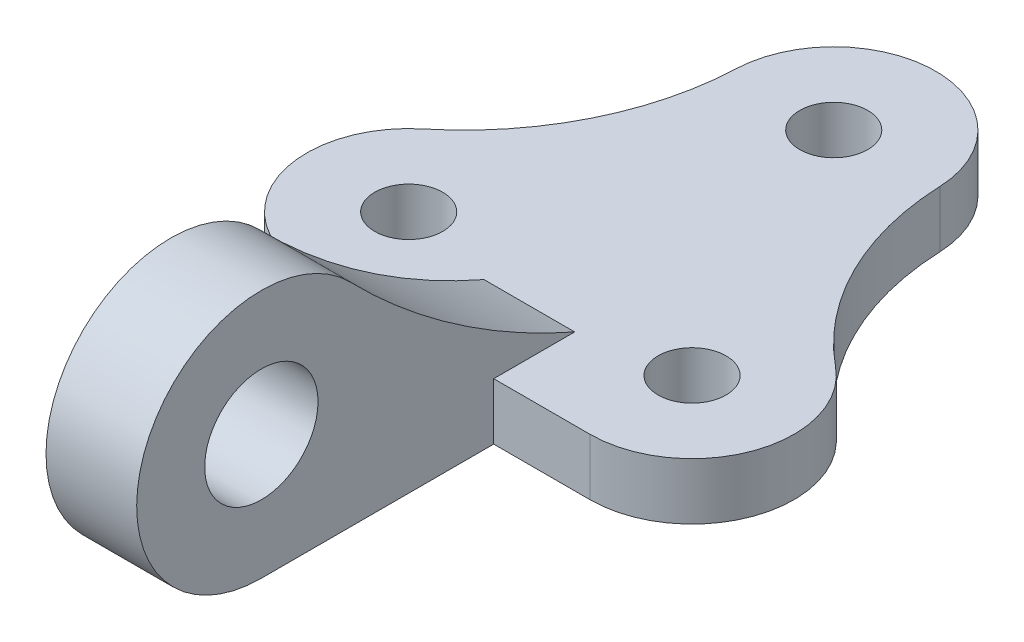
ISO-10303-21;
HEADER;
FILE_DESCRIPTION(('STEP AP214'),'2;1');
FILE_NAME('part.step','',(''),(''),'','','');
FILE_SCHEMA(('AUTOMOTIVE_DESIGN { 1 0 10303 214 1 1 1 1 }'));
ENDSEC;
DATA;
#1=APPLICATION_CONTEXT('core data for automotive mechanical design processes');
#2=APPLICATION_PROTOCOL_DEFINITION('international standard','automotive_design',2000,#1);
#3=PRODUCT_CONTEXT('',#1,'mechanical');
#4=PRODUCT('Part','Part','',(#3));
#5=PRODUCT_RELATED_PRODUCT_CATEGORY('part','',(#4));
#6=PRODUCT_DEFINITION_FORMATION('','',#4);
#7=PRODUCT_DEFINITION_CONTEXT('part definition',#1,'design');
#8=PRODUCT_DEFINITION('design','',#6,#7);
#9=PRODUCT_DEFINITION_SHAPE('','',#8);
#10=(LENGTH_UNIT() NAMED_UNIT(*) SI_UNIT(.MILLI.,.METRE.));
#11=(NAMED_UNIT(*) PLANE_ANGLE_UNIT() SI_UNIT($,.RADIAN.));
#12=(NAMED_UNIT(*) SI_UNIT($,.STERADIAN.) SOLID_ANGLE_UNIT());
#13=UNCERTAINTY_MEASURE_WITH_UNIT(LENGTH_MEASURE(1.E-05),#10,'distance_accuracy_value','');
#14=(GEOMETRIC_REPRESENTATION_CONTEXT(3) GLOBAL_UNCERTAINTY_ASSIGNED_CONTEXT((#13)) GLOBAL_UNIT_ASSIGNED_CONTEXT((#10,
#11,#12)) REPRESENTATION_CONTEXT('',''));
#15=CARTESIAN_POINT('',(0.,0.,0.));
#16=DIRECTION('',(0.,0.,1.));
#17=DIRECTION('',(1.,0.,0.));
#18=AXIS2_PLACEMENT_3D('',#15,#16,#17);
#19=CARTESIAN_POINT('',(-67.9454687057473,10.,-2.72273435287363));
#20=DIRECTION('',(0.,-1.,0.));
#21=DIRECTION('',(0.,0.,-1.));
#22=AXIS2_PLACEMENT_3D('',#19,#20,#21);
#23=PLANE('',#22);
#24=CARTESIAN_POINT('',(-67.9454687057473,10.,-2.72273435287363));
#25=DIRECTION('',(0.,-1.,0.));
#26=DIRECTION('',(0.,0.,-1.));
#27=AXIS2_PLACEMENT_3D('',#24,#25,#26);
#28=CIRCLE('',#27,50.);
#29=CARTESIAN_POINT('',(-17.985565245639,10.,-0.720723799290078));
#30=VERTEX_POINT('',#29);
#31=CARTESIAN_POINT('',(-36.3679181868154,10.,36.0439820830629));
#32=VERTEX_POINT('',#31);
#33=EDGE_CURVE('E144',#30,#32,#28,.T.);
#34=ORIENTED_EDGE('',*,*,#33,.T.);
#35=CARTESIAN_POINT('',(-25.,10.,50.));
#36=DIRECTION('',(0.,1.,0.));
#37=DIRECTION('',(0.,0.,1.));
#38=AXIS2_PLACEMENT_3D('',#35,#36,#37);
#39=CIRCLE('',#38,18.);
#40=CARTESIAN_POINT('',(-25.,10.,68.));
#41=VERTEX_POINT('',#40);
#42=EDGE_CURVE('E100',#32,#41,#39,.T.);
#43=ORIENTED_EDGE('',*,*,#42,.T.);
#44=DIRECTION('',(1.,0.,0.));
#45=VECTOR('',#44,1.);
#46=CARTESIAN_POINT('',(-7.99999999999999,10.,68.));
#47=LINE('',#46,#45);
#48=CARTESIAN_POINT('',(-7.99999999999999,10.,68.));
#49=VERTEX_POINT('',#48);
#50=EDGE_CURVE('E165',#41,#49,#47,.T.);
#51=ORIENTED_EDGE('',*,*,#50,.T.);
#52=DIRECTION('',(0.,0.,-1.));
#53=VECTOR('',#52,1.);
#54=CARTESIAN_POINT('',(-7.99999999999999,10.,68.));
#55=LINE('',#54,#53);
#56=CARTESIAN_POINT('',(-8.,10.,53.71));
#57=VERTEX_POINT('',#56);
#58=EDGE_CURVE('E212',#49,#57,#55,.T.);
#59=ORIENTED_EDGE('',*,*,#58,.T.);
#60=DIRECTION('',(1.,0.,0.));
#61=VECTOR('',#60,1.);
#62=CARTESIAN_POINT('',(-7.99999999999999,10.,53.71));
#63=LINE('',#62,#61);
#64=CARTESIAN_POINT('',(8.,10.,53.71));
#65=VERTEX_POINT('',#64);
#66=EDGE_CURVE('E220',#57,#65,#63,.T.);
#67=ORIENTED_EDGE('',*,*,#66,.T.);
#68=DIRECTION('',(0.,0.,1.));
#69=VECTOR('',#68,1.);
#70=CARTESIAN_POINT('',(8.00000000000001,10.,68.));
#71=LINE('',#70,#69);
#72=CARTESIAN_POINT('',(8.,10.,68.));
#73=VERTEX_POINT('',#72);
#74=EDGE_CURVE('E219',#65,#73,#71,.T.);
#75=ORIENTED_EDGE('',*,*,#74,.T.);
#76=DIRECTION('',(1.,0.,0.));
#77=VECTOR('',#76,1.);
#78=CARTESIAN_POINT('',(25.,10.,68.));
#79=LINE('',#78,#77);
#80=CARTESIAN_POINT('',(25.,10.,68.));
#81=VERTEX_POINT('',#80);
#82=EDGE_CURVE('E114',#73,#81,#79,.T.);
#83=ORIENTED_EDGE('',*,*,#82,.T.);
#84=CARTESIAN_POINT('',(25.,10.,50.));
#85=DIRECTION('',(0.,1.,0.));
#86=DIRECTION('',(0.,0.,1.));
#87=AXIS2_PLACEMENT_3D('',#84,#85,#86);
#88=CIRCLE('',#87,18.);
#89=CARTESIAN_POINT('',(36.3679181868155,10.,36.0439820830629));
#90=VERTEX_POINT('',#89);
#91=EDGE_CURVE('E106',#81,#90,#88,.T.);
#92=ORIENTED_EDGE('',*,*,#91,.T.);
#93=CARTESIAN_POINT('',(67.9454687057473,10.,-2.72273435287364));
#94=DIRECTION('',(0.,-1.,0.));
#95=DIRECTION('',(0.,0.,1.));
#96=AXIS2_PLACEMENT_3D('',#93,#94,#95);
#97=CIRCLE('',#96,50.);
#98=CARTESIAN_POINT('',(17.985565245639,10.,-0.720723799290081));
#99=VERTEX_POINT('',#98);
#100=EDGE_CURVE('E109',#90,#99,#97,.T.);
#101=ORIENTED_EDGE('',*,*,#100,.T.);
#102=CARTESIAN_POINT('',(0.,10.,0.));
#103=DIRECTION('',(0.,1.,0.));
#104=DIRECTION('',(0.,0.,1.));
#105=AXIS2_PLACEMENT_3D('',#102,#103,#104);
#106=CIRCLE('',#105,18.);
#107=EDGE_CURVE('E57',#99,#30,#106,.T.);
#108=ORIENTED_EDGE('',*,*,#107,.T.);
#109=EDGE_LOOP('',(#34,#43,#51,#59,#67,#75,#83,#92,#101,#108));
#110=FACE_BOUND('',#109,.T.);
#111=CARTESIAN_POINT('',(0.,10.,0.));
#112=DIRECTION('',(0.,1.,0.));
#113=DIRECTION('',(0.,0.,1.));
#114=AXIS2_PLACEMENT_3D('',#111,#112,#113);
#115=CIRCLE('',#114,6.);
#116=CARTESIAN_POINT('',(0.,10.,6.));
#117=VERTEX_POINT('',#116);
#118=EDGE_CURVE('E132',#117,#117,#115,.T.);
#119=ORIENTED_EDGE('',*,*,#118,.F.);
#120=EDGE_LOOP('',(#119));
#121=FACE_BOUND('',#120,.T.);
#122=CARTESIAN_POINT('',(-25.,10.,50.));
#123=DIRECTION('',(0.,1.,0.));
#124=DIRECTION('',(0.,0.,1.));
#125=AXIS2_PLACEMENT_3D('',#122,#123,#124);
#126=CIRCLE('',#125,6.00000000000001);
#127=CARTESIAN_POINT('',(-25.,10.,56.));
#128=VERTEX_POINT('',#127);
#129=EDGE_CURVE('E203',#128,#128,#126,.T.);
#130=ORIENTED_EDGE('',*,*,#129,.F.);
#131=EDGE_LOOP('',(#130));
#132=FACE_BOUND('',#131,.T.);
#133=CARTESIAN_POINT('',(25.,10.,50.));
#134=DIRECTION('',(0.,1.,0.));
#135=DIRECTION('',(0.,0.,1.));
#136=AXIS2_PLACEMENT_3D('',#133,#134,#135);
#137=CIRCLE('',#136,5.99999999999999);
#138=CARTESIAN_POINT('',(25.,10.,56.));
#139=VERTEX_POINT('',#138);
#140=EDGE_CURVE('E194',#139,#139,#137,.T.);
#141=ORIENTED_EDGE('',*,*,#140,.F.);
#142=EDGE_LOOP('',(#141));
#143=FACE_BOUND('',#142,.T.);
#144=ADVANCED_FACE('F39',(#110,#121,#132,#143),#23,.F.);
#145=CARTESIAN_POINT('',(-67.9454687057473,0.,-2.72273435287363));
#146=DIRECTION('',(0.,-1.,0.));
#147=DIRECTION('',(0.,0.,-1.));
#148=AXIS2_PLACEMENT_3D('',#145,#146,#147);
#149=PLANE('',#148);
#150=CARTESIAN_POINT('',(-25.,0.,50.));
#151=DIRECTION('',(0.,1.,0.));
#152=DIRECTION('',(0.,0.,1.));
#153=AXIS2_PLACEMENT_3D('',#150,#151,#152);
#154=CIRCLE('',#153,6.00000000000001);
#155=CARTESIAN_POINT('',(-25.,0.,56.));
#156=VERTEX_POINT('',#155);
#157=EDGE_CURVE('E196',#156,#156,#154,.T.);
#158=ORIENTED_EDGE('',*,*,#157,.T.);
#159=EDGE_LOOP('',(#158));
#160=FACE_BOUND('',#159,.T.);
#161=CARTESIAN_POINT('',(-67.9454687057473,0.,-2.72273435287363));
#162=DIRECTION('',(0.,-1.,0.));
#163=DIRECTION('',(0.,0.,-1.));
#164=AXIS2_PLACEMENT_3D('',#161,#162,#163);
#165=CIRCLE('',#164,50.);
#166=CARTESIAN_POINT('',(-17.985565245639,0.,-0.720723799290078));
#167=VERTEX_POINT('',#166);
#168=CARTESIAN_POINT('',(-36.3679181868154,0.,36.0439820830629));
#169=VERTEX_POINT('',#168);
#170=EDGE_CURVE('E134',#167,#169,#165,.T.);
#171=ORIENTED_EDGE('',*,*,#170,.F.);
#172=CARTESIAN_POINT('',(0.,0.,0.));
#173=DIRECTION('',(0.,1.,0.));
#174=DIRECTION('',(0.,0.,1.));
#175=AXIS2_PLACEMENT_3D('',#172,#173,#174);
#176=CIRCLE('',#175,18.);
#177=CARTESIAN_POINT('',(17.985565245639,0.,-0.720723799290081));
#178=VERTEX_POINT('',#177);
#179=EDGE_CURVE('E90',#178,#167,#176,.T.);
#180=ORIENTED_EDGE('',*,*,#179,.F.);
#181=CARTESIAN_POINT('',(67.9454687057473,0.,-2.72273435287364));
#182=DIRECTION('',(0.,-1.,0.));
#183=DIRECTION('',(0.,0.,1.));
#184=AXIS2_PLACEMENT_3D('',#181,#182,#183);
#185=CIRCLE('',#184,50.);
#186=CARTESIAN_POINT('',(36.3679181868155,0.,36.0439820830629));
#187=VERTEX_POINT('',#186);
#188=EDGE_CURVE('E82',#187,#178,#185,.T.);
#189=ORIENTED_EDGE('',*,*,#188,.F.);
#190=CARTESIAN_POINT('',(25.,0.,50.));
#191=DIRECTION('',(0.,1.,0.));
#192=DIRECTION('',(0.,0.,1.));
#193=AXIS2_PLACEMENT_3D('',#190,#191,#192);
#194=CIRCLE('',#193,18.);
#195=CARTESIAN_POINT('',(25.,0.,68.));
#196=VERTEX_POINT('',#195);
#197=EDGE_CURVE('E121',#196,#187,#194,.T.);
#198=ORIENTED_EDGE('',*,*,#197,.F.);
#199=DIRECTION('',(1.,0.,0.));
#200=VECTOR('',#199,1.);
#201=CARTESIAN_POINT('',(25.,0.,68.));
#202=LINE('',#201,#200);
#203=CARTESIAN_POINT('',(8.00000000000001,0.,68.));
#204=VERTEX_POINT('',#203);
#205=EDGE_CURVE('E139',#204,#196,#202,.T.);
#206=ORIENTED_EDGE('',*,*,#205,.F.);
#207=DIRECTION('',(0.,0.,-1.));
#208=VECTOR('',#207,1.);
#209=CARTESIAN_POINT('',(8.,0.,109.));
#210=LINE('',#209,#208);
#211=CARTESIAN_POINT('',(8.,0.,109.));
#212=VERTEX_POINT('',#211);
#213=EDGE_CURVE('E293',#212,#204,#210,.T.);
#214=ORIENTED_EDGE('',*,*,#213,.F.);
#215=DIRECTION('',(-1.,0.,0.));
#216=VECTOR('',#215,1.);
#217=CARTESIAN_POINT('',(8.,0.,109.));
#218=LINE('',#217,#216);
#219=CARTESIAN_POINT('',(-8.,0.,109.));
#220=VERTEX_POINT('',#219);
#221=EDGE_CURVE('E173',#212,#220,#218,.T.);
#222=ORIENTED_EDGE('',*,*,#221,.T.);
#223=DIRECTION('',(0.,0.,-1.));
#224=VECTOR('',#223,1.);
#225=CARTESIAN_POINT('',(-8.,0.,109.));
#226=LINE('',#225,#224);
#227=CARTESIAN_POINT('',(-8.,0.,68.));
#228=VERTEX_POINT('',#227);
#229=EDGE_CURVE('E168',#220,#228,#226,.T.);
#230=ORIENTED_EDGE('',*,*,#229,.T.);
#231=DIRECTION('',(1.,0.,0.));
#232=VECTOR('',#231,1.);
#233=CARTESIAN_POINT('',(-7.99999999999999,0.,68.));
#234=LINE('',#233,#232);
#235=CARTESIAN_POINT('',(-25.,0.,68.));
#236=VERTEX_POINT('',#235);
#237=EDGE_CURVE('E140',#236,#228,#234,.T.);
#238=ORIENTED_EDGE('',*,*,#237,.F.);
#239=CARTESIAN_POINT('',(-25.,0.,50.));
#240=DIRECTION('',(0.,1.,0.));
#241=DIRECTION('',(0.,0.,1.));
#242=AXIS2_PLACEMENT_3D('',#239,#240,#241);
#243=CIRCLE('',#242,18.);
#244=EDGE_CURVE('E133',#169,#236,#243,.T.);
#245=ORIENTED_EDGE('',*,*,#244,.F.);
#246=EDGE_LOOP('',(#171,#180,#189,#198,#206,#214,#222,#230,#238,#245));
#247=FACE_BOUND('',#246,.T.);
#248=CARTESIAN_POINT('',(0.,0.,0.));
#249=DIRECTION('',(0.,1.,0.));
#250=DIRECTION('',(0.,0.,1.));
#251=AXIS2_PLACEMENT_3D('',#248,#249,#250);
#252=CIRCLE('',#251,6.);
#253=CARTESIAN_POINT('',(0.,0.,6.));
#254=VERTEX_POINT('',#253);
#255=EDGE_CURVE('E204',#254,#254,#252,.T.);
#256=ORIENTED_EDGE('',*,*,#255,.T.);
#257=EDGE_LOOP('',(#256));
#258=FACE_BOUND('',#257,.T.);
#259=CARTESIAN_POINT('',(25.,0.,50.));
#260=DIRECTION('',(0.,1.,0.));
#261=DIRECTION('',(0.,0.,1.));
#262=AXIS2_PLACEMENT_3D('',#259,#260,#261);
#263=CIRCLE('',#262,5.99999999999999);
#264=CARTESIAN_POINT('',(25.,0.,56.));
#265=VERTEX_POINT('',#264);
#266=EDGE_CURVE('E193',#265,#265,#263,.T.);
#267=ORIENTED_EDGE('',*,*,#266,.T.);
#268=EDGE_LOOP('',(#267));
#269=FACE_BOUND('',#268,.T.);
#270=ADVANCED_FACE('F167',(#160,#247,#258,#269),#149,.T.);
#271=CARTESIAN_POINT('',(-67.9454687057473,10.,-2.72273435287363));
#272=DIRECTION('',(0.,-1.,0.));
#273=DIRECTION('',(0.,0.,-1.));
#274=AXIS2_PLACEMENT_3D('',#271,#272,#273);
#275=CYLINDRICAL_SURFACE('',#274,50.);
#276=ORIENTED_EDGE('',*,*,#170,.T.);
#277=DIRECTION('',(0.,-1.,0.));
#278=VECTOR('',#277,1.);
#279=CARTESIAN_POINT('',(-36.3679181868154,10.,36.0439820830629));
#280=LINE('',#279,#278);
#281=EDGE_CURVE('E11',#32,#169,#280,.T.);
#282=ORIENTED_EDGE('',*,*,#281,.F.);
#283=ORIENTED_EDGE('',*,*,#33,.F.);
#284=DIRECTION('',(0.,-1.,0.));
#285=VECTOR('',#284,1.);
#286=CARTESIAN_POINT('',(-17.985565245639,10.,-0.720723799290078));
#287=LINE('',#286,#285);
#288=EDGE_CURVE('E130',#30,#167,#287,.T.);
#289=ORIENTED_EDGE('',*,*,#288,.T.);
#290=EDGE_LOOP('',(#276,#282,#283,#289));
#291=FACE_BOUND('',#290,.T.);
#292=ADVANCED_FACE('F41',(#291),#275,.F.);
#293=CARTESIAN_POINT('',(-25.,10.,50.));
#294=DIRECTION('',(0.,-1.,0.));
#295=DIRECTION('',(0.,0.,-1.));
#296=AXIS2_PLACEMENT_3D('',#293,#294,#295);
#297=CYLINDRICAL_SURFACE('',#296,18.);
#298=ORIENTED_EDGE('',*,*,#244,.T.);
#299=DIRECTION('',(0.,-1.,0.));
#300=VECTOR('',#299,1.);
#301=CARTESIAN_POINT('',(-25.,10.,68.));
#302=LINE('',#301,#300);
#303=EDGE_CURVE('E48',#41,#236,#302,.T.);
#304=ORIENTED_EDGE('',*,*,#303,.F.);
#305=ORIENTED_EDGE('',*,*,#42,.F.);
#306=ORIENTED_EDGE('',*,*,#281,.T.);
#307=EDGE_LOOP('',(#298,#304,#305,#306));
#308=FACE_BOUND('',#307,.T.);
#309=ADVANCED_FACE('F343',(#308),#297,.T.);
#310=CARTESIAN_POINT('',(-7.99999999999999,10.,68.));
#311=DIRECTION('',(0.,0.,-1.));
#312=DIRECTION('',(-1.,0.,0.));
#313=AXIS2_PLACEMENT_3D('',#310,#311,#312);
#314=PLANE('',#313);
#315=ORIENTED_EDGE('',*,*,#237,.T.);
#316=DIRECTION('',(0.,-1.,0.));
#317=VECTOR('',#316,1.);
#318=CARTESIAN_POINT('',(-7.99999999999999,10.,68.));
#319=LINE('',#318,#317);
#320=EDGE_CURVE('E155',#49,#228,#319,.T.);
#321=ORIENTED_EDGE('',*,*,#320,.F.);
#322=ORIENTED_EDGE('',*,*,#50,.F.);
#323=ORIENTED_EDGE('',*,*,#303,.T.);
#324=EDGE_LOOP('',(#315,#321,#322,#323));
#325=FACE_BOUND('',#324,.T.);
#326=ADVANCED_FACE('F158',(#325),#314,.F.);
#327=CARTESIAN_POINT('',(25.,10.,68.));
#328=DIRECTION('',(0.,0.,-1.));
#329=DIRECTION('',(-1.,0.,0.));
#330=AXIS2_PLACEMENT_3D('',#327,#328,#329);
#331=PLANE('',#330);
#332=ORIENTED_EDGE('',*,*,#205,.T.);
#333=DIRECTION('',(0.,-1.,0.));
#334=VECTOR('',#333,1.);
#335=CARTESIAN_POINT('',(25.,10.,68.));
#336=LINE('',#335,#334);
#337=EDGE_CURVE('E125',#81,#196,#336,.T.);
#338=ORIENTED_EDGE('',*,*,#337,.F.);
#339=ORIENTED_EDGE('',*,*,#82,.F.);
#340=DIRECTION('',(0.,-1.,0.));
#341=VECTOR('',#340,1.);
#342=CARTESIAN_POINT('',(8.00000000000001,10.,68.));
#343=LINE('',#342,#341);
#344=EDGE_CURVE('E149',#73,#204,#343,.T.);
#345=ORIENTED_EDGE('',*,*,#344,.T.);
#346=EDGE_LOOP('',(#332,#338,#339,#345));
#347=FACE_BOUND('',#346,.T.);
#348=ADVANCED_FACE('F231',(#347),#331,.F.);
#349=CARTESIAN_POINT('',(25.,10.,50.));
#350=DIRECTION('',(0.,-1.,0.));
#351=DIRECTION('',(0.,0.,-1.));
#352=AXIS2_PLACEMENT_3D('',#349,#350,#351);
#353=CYLINDRICAL_SURFACE('',#352,18.);
#354=ORIENTED_EDGE('',*,*,#197,.T.);
#355=DIRECTION('',(0.,-1.,0.));
#356=VECTOR('',#355,1.);
#357=CARTESIAN_POINT('',(36.3679181868155,10.,36.0439820830629));
#358=LINE('',#357,#356);
#359=EDGE_CURVE('E120',#90,#187,#358,.T.);
#360=ORIENTED_EDGE('',*,*,#359,.F.);
#361=ORIENTED_EDGE('',*,*,#91,.F.);
#362=ORIENTED_EDGE('',*,*,#337,.T.);
#363=EDGE_LOOP('',(#354,#360,#361,#362));
#364=FACE_BOUND('',#363,.T.);
#365=ADVANCED_FACE('F118',(#364),#353,.T.);
#366=CARTESIAN_POINT('',(67.9454687057473,10.,-2.72273435287364));
#367=DIRECTION('',(0.,-1.,0.));
#368=DIRECTION('',(0.,0.,-1.));
#369=AXIS2_PLACEMENT_3D('',#366,#367,#368);
#370=CYLINDRICAL_SURFACE('',#369,50.);
#371=ORIENTED_EDGE('',*,*,#188,.T.);
#372=DIRECTION('',(0.,-1.,0.));
#373=VECTOR('',#372,1.);
#374=CARTESIAN_POINT('',(17.985565245639,10.,-0.720723799290081));
#375=LINE('',#374,#373);
#376=EDGE_CURVE('E122',#99,#178,#375,.T.);
#377=ORIENTED_EDGE('',*,*,#376,.F.);
#378=ORIENTED_EDGE('',*,*,#100,.F.);
#379=ORIENTED_EDGE('',*,*,#359,.T.);
#380=EDGE_LOOP('',(#371,#377,#378,#379));
#381=FACE_BOUND('',#380,.T.);
#382=ADVANCED_FACE('F124',(#381),#370,.F.);
#383=CARTESIAN_POINT('',(0.,10.,0.));
#384=DIRECTION('',(0.,-1.,0.));
#385=DIRECTION('',(0.,0.,-1.));
#386=AXIS2_PLACEMENT_3D('',#383,#384,#385);
#387=CYLINDRICAL_SURFACE('',#386,18.);
#388=ORIENTED_EDGE('',*,*,#179,.T.);
#389=ORIENTED_EDGE('',*,*,#288,.F.);
#390=ORIENTED_EDGE('',*,*,#107,.F.);
#391=ORIENTED_EDGE('',*,*,#376,.T.);
#392=EDGE_LOOP('',(#388,#389,#390,#391));
#393=FACE_BOUND('',#392,.T.);
#394=ADVANCED_FACE('F237',(#393),#387,.T.);
#395=CARTESIAN_POINT('',(0.,10.,0.));
#396=DIRECTION('',(0.,-1.,0.));
#397=DIRECTION('',(0.,0.,-1.));
#398=AXIS2_PLACEMENT_3D('',#395,#396,#397);
#399=CYLINDRICAL_SURFACE('',#398,6.);
#400=ORIENTED_EDGE('',*,*,#118,.T.);
#401=EDGE_LOOP('',(#400));
#402=FACE_BOUND('',#401,.T.);
#403=ORIENTED_EDGE('',*,*,#255,.F.);
#404=EDGE_LOOP('',(#403));
#405=FACE_BOUND('',#404,.T.);
#406=ADVANCED_FACE('F236',(#402,#405),#399,.F.);
#407=CARTESIAN_POINT('',(-25.,10.,50.));
#408=DIRECTION('',(0.,-1.,0.));
#409=DIRECTION('',(0.,0.,-1.));
#410=AXIS2_PLACEMENT_3D('',#407,#408,#409);
#411=CYLINDRICAL_SURFACE('',#410,6.00000000000001);
#412=ORIENTED_EDGE('',*,*,#129,.T.);
#413=EDGE_LOOP('',(#412));
#414=FACE_BOUND('',#413,.T.);
#415=ORIENTED_EDGE('',*,*,#157,.F.);
#416=EDGE_LOOP('',(#415));
#417=FACE_BOUND('',#416,.T.);
#418=ADVANCED_FACE('F243',(#414,#417),#411,.F.);
#419=CARTESIAN_POINT('',(25.,10.,50.));
#420=DIRECTION('',(0.,-1.,0.));
#421=DIRECTION('',(0.,0.,-1.));
#422=AXIS2_PLACEMENT_3D('',#419,#420,#421);
#423=CYLINDRICAL_SURFACE('',#422,5.99999999999999);
#424=ORIENTED_EDGE('',*,*,#140,.T.);
#425=EDGE_LOOP('',(#424));
#426=FACE_BOUND('',#425,.T.);
#427=ORIENTED_EDGE('',*,*,#266,.F.);
#428=EDGE_LOOP('',(#427));
#429=FACE_BOUND('',#428,.T.);
#430=ADVANCED_FACE('F259',(#426,#429),#423,.F.);
#431=CARTESIAN_POINT('',(-8.,22.,109.));
#432=DIRECTION('',(1.,0.,0.));
#433=DIRECTION('',(0.,0.,-1.));
#434=AXIS2_PLACEMENT_3D('',#431,#432,#433);
#435=PLANE('',#434);
#436=CARTESIAN_POINT('',(-8.,22.,109.));
#437=DIRECTION('',(1.,0.,0.));
#438=DIRECTION('',(0.,0.,-1.));
#439=AXIS2_PLACEMENT_3D('',#436,#437,#438);
#440=CIRCLE('',#439,9.99999999999999);
#441=CARTESIAN_POINT('',(-8.,22.,99.));
#442=VERTEX_POINT('',#441);
#443=EDGE_CURVE('E288',#442,#442,#440,.T.);
#444=ORIENTED_EDGE('',*,*,#443,.T.);
#445=EDGE_LOOP('',(#444));
#446=FACE_BOUND('',#445,.T.);
#447=CARTESIAN_POINT('',(-8.,124.551548704628,3.68058176061609));
#448=DIRECTION('',(-1.,0.,0.));
#449=DIRECTION('',(0.,0.,-1.));
#450=AXIS2_PLACEMENT_3D('',#447,#448,#449);
#451=CIRCLE('',#450,125.);
#452=CARTESIAN_POINT('',(-8.,37.347850826543,93.2379101954664));
#453=VERTEX_POINT('',#452);
#454=EDGE_CURVE('E178',#57,#453,#451,.T.);
#455=ORIENTED_EDGE('',*,*,#454,.F.);
#456=ORIENTED_EDGE('',*,*,#58,.F.);
#457=ORIENTED_EDGE('',*,*,#320,.T.);
#458=ORIENTED_EDGE('',*,*,#229,.F.);
#459=CARTESIAN_POINT('',(-8.,22.,109.));
#460=DIRECTION('',(1.,0.,0.));
#461=DIRECTION('',(0.,0.,-1.));
#462=AXIS2_PLACEMENT_3D('',#459,#460,#461);
#463=CIRCLE('',#462,22.);
#464=EDGE_CURVE('E179',#453,#220,#463,.T.);
#465=ORIENTED_EDGE('',*,*,#464,.F.);
#466=EDGE_LOOP('',(#455,#456,#457,#458,#465));
#467=FACE_BOUND('',#466,.T.);
#468=ADVANCED_FACE('F265',(#446,#467),#435,.F.);
#469=CARTESIAN_POINT('',(8.,22.,109.));
#470=DIRECTION('',(1.,0.,0.));
#471=DIRECTION('',(0.,0.,-1.));
#472=AXIS2_PLACEMENT_3D('',#469,#470,#471);
#473=PLANE('',#472);
#474=CARTESIAN_POINT('',(8.,22.,109.));
#475=DIRECTION('',(1.,0.,0.));
#476=DIRECTION('',(0.,0.,-1.));
#477=AXIS2_PLACEMENT_3D('',#474,#475,#476);
#478=CIRCLE('',#477,9.99999999999999);
#479=CARTESIAN_POINT('',(8.,22.,99.));
#480=VERTEX_POINT('',#479);
#481=EDGE_CURVE('E183',#480,#480,#478,.T.);
#482=ORIENTED_EDGE('',*,*,#481,.F.);
#483=EDGE_LOOP('',(#482));
#484=FACE_BOUND('',#483,.T.);
#485=ORIENTED_EDGE('',*,*,#74,.F.);
#486=CARTESIAN_POINT('',(8.,124.551548704628,3.68058176061609));
#487=DIRECTION('',(-1.,0.,0.));
#488=DIRECTION('',(0.,0.,-1.));
#489=AXIS2_PLACEMENT_3D('',#486,#487,#488);
#490=CIRCLE('',#489,125.);
#491=CARTESIAN_POINT('',(8.,37.347850826543,93.2379101954664));
#492=VERTEX_POINT('',#491);
#493=EDGE_CURVE('E195',#65,#492,#490,.T.);
#494=ORIENTED_EDGE('',*,*,#493,.T.);
#495=CARTESIAN_POINT('',(8.,22.,109.));
#496=DIRECTION('',(1.,0.,0.));
#497=DIRECTION('',(0.,0.,-1.));
#498=AXIS2_PLACEMENT_3D('',#495,#496,#497);
#499=CIRCLE('',#498,22.);
#500=EDGE_CURVE('E181',#492,#212,#499,.T.);
#501=ORIENTED_EDGE('',*,*,#500,.T.);
#502=ORIENTED_EDGE('',*,*,#213,.T.);
#503=ORIENTED_EDGE('',*,*,#344,.F.);
#504=EDGE_LOOP('',(#485,#494,#501,#502,#503));
#505=FACE_BOUND('',#504,.T.);
#506=ADVANCED_FACE('F268',(#484,#505),#473,.T.);
#507=CARTESIAN_POINT('',(8.,22.,109.));
#508=DIRECTION('',(-1.,0.,0.));
#509=DIRECTION('',(0.,0.,1.));
#510=AXIS2_PLACEMENT_3D('',#507,#508,#509);
#511=CYLINDRICAL_SURFACE('',#510,22.);
#512=ORIENTED_EDGE('',*,*,#464,.T.);
#513=ORIENTED_EDGE('',*,*,#221,.F.);
#514=ORIENTED_EDGE('',*,*,#500,.F.);
#515=DIRECTION('',(-1.,0.,0.));
#516=VECTOR('',#515,1.);
#517=CARTESIAN_POINT('',(8.,37.347850826543,93.2379101954664));
#518=LINE('',#517,#516);
#519=EDGE_CURVE('E188',#492,#453,#518,.T.);
#520=ORIENTED_EDGE('',*,*,#519,.T.);
#521=EDGE_LOOP('',(#512,#513,#514,#520));
#522=FACE_BOUND('',#521,.T.);
#523=ADVANCED_FACE('F262',(#522),#511,.T.);
#524=CARTESIAN_POINT('',(8.,124.551548704628,3.68058176061609));
#525=DIRECTION('',(-1.,0.,0.));
#526=DIRECTION('',(0.,0.,1.));
#527=AXIS2_PLACEMENT_3D('',#524,#525,#526);
#528=CYLINDRICAL_SURFACE('',#527,125.);
#529=ORIENTED_EDGE('',*,*,#454,.T.);
#530=ORIENTED_EDGE('',*,*,#519,.F.);
#531=ORIENTED_EDGE('',*,*,#493,.F.);
#532=ORIENTED_EDGE('',*,*,#66,.F.);
#533=EDGE_LOOP('',(#529,#530,#531,#532));
#534=FACE_BOUND('',#533,.T.);
#535=ADVANCED_FACE('F270',(#534),#528,.F.);
#536=CARTESIAN_POINT('',(8.,22.,109.));
#537=DIRECTION('',(-1.,0.,0.));
#538=DIRECTION('',(0.,0.,1.));
#539=AXIS2_PLACEMENT_3D('',#536,#537,#538);
#540=CYLINDRICAL_SURFACE('',#539,9.99999999999999);
#541=ORIENTED_EDGE('',*,*,#481,.T.);
#542=EDGE_LOOP('',(#541));
#543=FACE_BOUND('',#542,.T.);
#544=ORIENTED_EDGE('',*,*,#443,.F.);
#545=EDGE_LOOP('',(#544));
#546=FACE_BOUND('',#545,.T.);
#547=ADVANCED_FACE('F275',(#543,#546),#540,.F.);
#548=CLOSED_SHELL('',(#144,#270,#292,#309,#326,#348,#365,#382,#394,#406,#418,#430,#468,#506,
#523,#535,#547));
#549=MANIFOLD_SOLID_BREP('B2',#548);
#550=ADVANCED_BREP_SHAPE_REPRESENTATION('',(#18,#549),#14);
#551=SHAPE_DEFINITION_REPRESENTATION(#9,#550);
ENDSEC;
END-ISO-10303-21;
